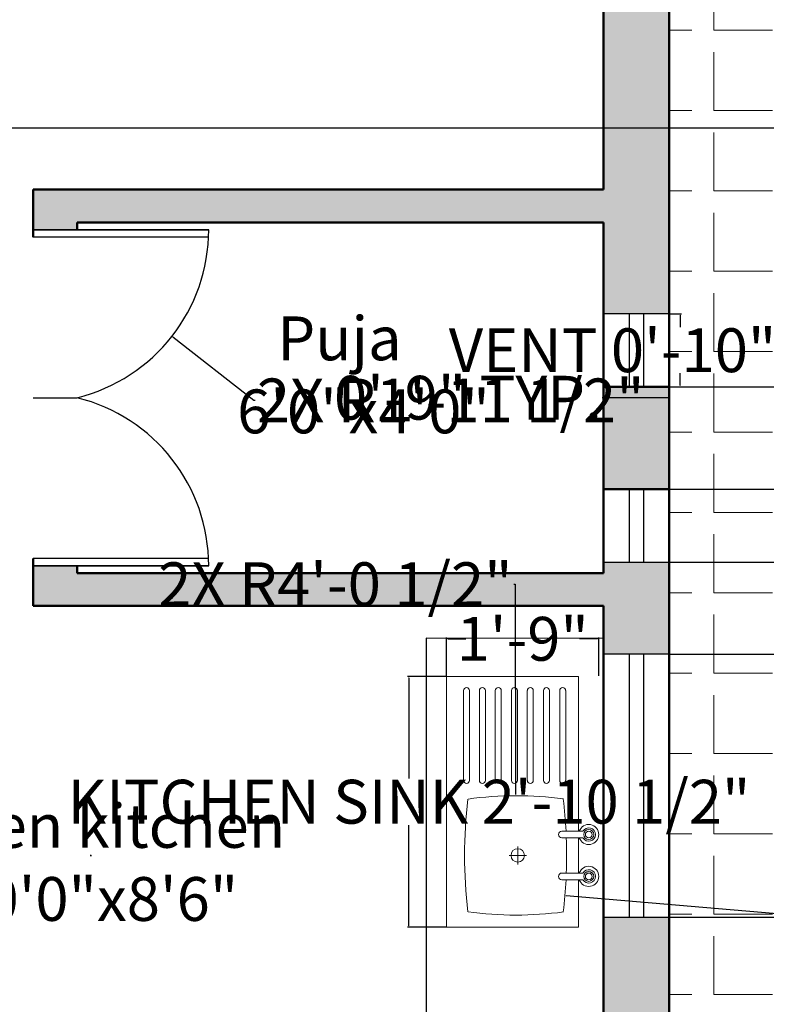
# Model space of a CAD drawing. Units: inches. Extents: x 1601 to 2080, y 5000 to 5589.
# Tile 5 of 11: x 1874 to 1976, y 5125 to 5259. Entities that reach past the tile are written whole.
import ezdxf

# ---------------------------------------------------------------- set-up
doc = ezdxf.new("R2010")
doc.units = ezdxf.units.IN
doc.header["$MEASUREMENT"] = 0
for name, color, linetype, lineweight in [('A-ANNO-DIMS', 2, 'Continuous', 18), ('A-AREA-IDEN', 7, 'Continuous', 25), ('A-COLS', 7, 'Continuous', 50), ('A-COLS-PATT', 18, 'Continuous', 13), ('A-DOOR', 3, 'Continuous', 25), ('A-FLOR-CASE', 8, 'Continuous', 25), ('A-FLOR-FIXT', 7, 'Continuous', 18), ('A-FLOR-PATT', 8, 'Continuous', 13), ('A-GLAZ', 4, 'Continuous', 25), ('A-WALL', 7, 'Continuous', 50), ('A-WALL-PATT', 241, 'Continuous', 13)]:
    doc.layers.add(name, color=color, linetype=linetype, lineweight=lineweight)
doc.styles.get("Standard").update_dxf_attribs({"font": 'arial.ttf'})
doc.dimstyles.get("Standard").update_dxf_attribs({"dimtxt": 6, "dimasz": 0.18, "dimexe": 0.18, "dimexo": 0.0625, "dimgap": 0.09, "dimtad": 0, "dimtih": 1, "dimtoh": 1, "dimdec": 1, "dimzin": 0, "dimdsep": 46, "dimlunit": 3, "dimtxsty": 'Standard', "dimcen": 0.09, "dimadec": 0, "dimazin": 0, "dimtfac": 1, "dimtdec": 1, "dimtofl": 0, "dimtmove": 0, "dimatfit": 3, "dimfxl": 1, "dimtolj": 1, "dimtzin": 0, "dimarcsym": 0})

# ---------------------------------------------------------------- blocks, each defined once
blk = doc.blocks.new('A$C799204C7')
for p, q in [((0, 34.2), (17.99, 34.2)), ((0, 0), (0, 34.2)), ((17.99, 13.08), (17.99, 34.2)), ((2.32, 20.01), (2.32, 32.27)), ((3.13, 20.01), (3.13, 32.27)), ((4.48, 20.01), (4.48, 32.27)), ((5.29, 20.01), (5.29, 32.27)), ((6.64, 20.01), (6.64, 32.27)), ((7.45, 20.01), (7.45, 32.27)), ((8.85, 20.01), (8.85, 32.27)), ((9.66, 20.01), (9.66, 32.27)), ((11.01, 20.01), (11.01, 32.27)), ((11.82, 20.01), (11.82, 32.27)), ((13.22, 20.01), (13.22, 32.27)), ((14.03, 20.01), (14.03, 32.27)), ((15.42, 20.01), (15.42, 32.27)), ((16.24, 20.01), (16.24, 32.27)), ((18.59, 13.08), (15.71, 13.08)), ((15.71, 12.17), (18.59, 12.17)), ((17.99, 7.36), (17.99, 12.17)), ((9.73, 11), (9.73, 8.54)), ((8.52, 9.77), (10.9, 9.77)), ((18.59, 7.36), (15.71, 7.36)), ((15.71, 6.45), (18.59, 6.45)), ((17.99, 0), (17.99, 6.45)), ((0, 0), (17.99, 0))]:
    blk.add_line(p, q)
for centre, radius in [((19.38, 12.62), 0.684), ((19.38, 12.62), 0.456), ((9.7, 9.77), 0.916), ((19.38, 6.91), 0.684), ((19.38, 6.91), 0.456)]:
    blk.add_circle(centre, radius)
for centre, radius, start, end in [((2.72, 32.27), 0.407, 0, 180), ((4.88, 32.27), 0.407, 0, 180), ((7.05, 32.27), 0.407, 0, 180), ((9.25, 32.27), 0.407, 0, 180), ((11.42, 32.27), 0.407, 0, 180), ((13.62, 32.27), 0.407, 0, 180), ((15.83, 32.27), 0.407, 0, 180), ((2.72, 20.01), 0.407, 180, 0), ((4.88, 20.01), 0.407, 180, 0), ((7.05, 20.01), 0.407, 180, 0), ((9.25, 20.01), 0.407, 180, 0), ((11.42, 20.01), 0.407, 180, 0), ((13.62, 20.01), 0.407, 180, 0), ((15.83, 20.01), 0.407, 180, 0), ((9.53, -30.19), 48.1, 82.3437, 97.8966), ((67.33, 9.77), 64.88, 173.1952, 186.8048), ((-48.51, 9.77), 64.88, 2.9208, 6.8048), ((19.38, 12.62), 1.37, 199.6514, 160.3603), ((19.38, 12.62), 0.911, 210.3431, 149.7554), ((15.71, 12.62), 0.456, 90, 270), ((-48.51, 9.77), 64.88, 357.8723, 2.115), ((19.38, 6.91), 1.37, 199.6514, 160.3603), ((15.71, 6.91), 0.456, 90, 270), ((19.38, 6.91), 0.911, 210.3431, 149.7554), ((-48.51, 9.77), 64.88, 353.1952, 357.0665), ((9.53, 49.73), 48.1, 262.1034, 277.6563)]:
    blk.add_arc(centre, radius, start, end)
blk = doc.blocks.new('WINDOW-36IN')
for p, q in [((0, 9), (0, 0)), ((36, 9), (0, 9)), ((36, 0), (36, 9)), ((36, 5.5), (0, 5.5)), ((0, 3.5), (36, 3.5)), ((0, 0), (36, 0))]:
    blk.add_line(p, q)
blk = doc.blocks.new('VENT-10IN')
for p, q in [((0, 10), (0, 0)), ((3.5, 10), (3.5, 0)), ((5.5, 0), (5.5, 10)), ((9, 0), (9, 10)), ((0, 0), (9, 0))]:
    blk.add_line(p, q)
blk = doc.blocks.new('*D33')
at = {"layer": 'A-ANNO-DIMS', "color": 0, "lineweight": -2, "transparency": 16777216}
for p, q in [((1962.97, 5219.2), (1964.59, 5219.2)), ((1964.41, 5219.02), (1964.41, 5217.35)), ((1964.41, 5209.38), (1964.41, 5211.04)), ((1962.97, 5209.2), (1964.59, 5209.2))]:
    blk.add_line(p, q, dxfattribs=at)
at = {"layer": 'A-ANNO-DIMS', "color": 0, "transparency": 16777216}
for points in [[(1964.38, 5219.02), (1964.44, 5219.02), (1964.41, 5219.2)], [(1964.38, 5209.38), (1964.44, 5209.38), (1964.41, 5209.2)]]:
    blk.add_solid(points, dxfattribs=at)
at = {"layer": 'Defpoints', "color": 0, "transparency": 16777216}
for p in [(1962.91, 5219.2), (1962.91, 5209.2), (1964.41, 5209.2)]:
    blk.add_point(p, dxfattribs=at)
at = {"layer": 'A-ANNO-DIMS', "color": 0, "transparency": 16777216, "insert": (1964.41, 5214.2), "char_height": 6, "attachment_point": 5}
blk.add_mtext('\\A1;VENT 0\'-10" TYP.', dxfattribs=at)
blk = doc.blocks.new('*D34')
at = {"layer": 'A-ANNO-DIMS', "color": 0, "lineweight": -2, "transparency": 16777216}
for p, q in [((1953.91, 5209.13), (1953.91, 5207.52)), ((1962.91, 5209.13), (1962.91, 5207.52)), ((1953.91, 5207.7), (1953.73, 5207.7)), ((1962.73, 5207.7), (1954.09, 5207.7))]:
    blk.add_line(p, q, dxfattribs=at)
at = {"layer": 'A-ANNO-DIMS', "color": 0, "transparency": 16777216}
for points in [[(1954.09, 5207.73), (1954.09, 5207.67), (1953.91, 5207.7)], [(1962.73, 5207.73), (1962.73, 5207.67), (1962.91, 5207.7)]]:
    blk.add_solid(points, dxfattribs=at)
at = {"layer": 'Defpoints', "color": 0, "transparency": 16777216}
for p in [(1953.91, 5209.2), (1962.91, 5209.2), (1953.91, 5207.7)]:
    blk.add_point(p, dxfattribs=at)
at = {"layer": 'A-ANNO-DIMS', "color": 0, "transparency": 16777216, "insert": (1935.35, 5207.7), "char_height": 6, "attachment_point": 5}
blk.add_mtext('\\A1;0\'-9" TYP.', dxfattribs=at)
blk = doc.blocks.new('*D35')
at = {"layer": 'A-ANNO-DIMS', "color": 0, "lineweight": -2, "transparency": 16777216}
for p, q in [((1932.38, 5169.56), (1927.11, 5169.56)), ((1927.29, 5169.38), (1927.29, 5155.59)), ((1927.29, 5135.43), (1927.29, 5149.21)), ((1932.38, 5135.25), (1927.11, 5135.25))]:
    blk.add_line(p, q, dxfattribs=at)
at = {"layer": 'A-ANNO-DIMS', "color": 0, "transparency": 16777216}
for points in [[(1927.26, 5169.38), (1927.32, 5169.38), (1927.29, 5169.56)], [(1927.26, 5135.43), (1927.32, 5135.43), (1927.29, 5135.25)]]:
    blk.add_solid(points, dxfattribs=at)
at = {"layer": 'Defpoints', "color": 0, "transparency": 16777216}
for p in [(1927.29, 5169.56), (1932.44, 5169.56), (1932.44, 5135.25)]:
    blk.add_point(p, dxfattribs=at)
at = {"layer": 'A-ANNO-DIMS', "color": 0, "transparency": 16777216, "insert": (1927.29, 5152.4), "char_height": 6, "attachment_point": 5}
blk.add_mtext('\\A1;KITCHEN SINK 2\'-10 1/2"', dxfattribs=at)
blk = doc.blocks.new('*D36')
at = {"layer": 'A-ANNO-DIMS', "color": 0, "lineweight": -2, "transparency": 16777216}
for p, q in [((1932.44, 5169.62), (1932.44, 5174.88)), ((1932.62, 5174.7), (1935.06, 5174.7)), ((1953.07, 5174.7), (1950.63, 5174.7)), ((1953.25, 5169.62), (1953.25, 5174.88))]:
    blk.add_line(p, q, dxfattribs=at)
at = {"layer": 'A-ANNO-DIMS', "color": 0, "transparency": 16777216}
for points in [[(1932.62, 5174.73), (1932.62, 5174.67), (1932.44, 5174.7)], [(1953.07, 5174.73), (1953.07, 5174.67), (1953.25, 5174.7)]]:
    blk.add_solid(points, dxfattribs=at)
at = {"layer": 'Defpoints', "color": 0, "transparency": 16777216}
for p in [(1953.25, 5174.7), (1932.44, 5169.56), (1953.25, 5169.56)]:
    blk.add_point(p, dxfattribs=at)
at = {"layer": 'A-ANNO-DIMS', "color": 0, "transparency": 16777216, "insert": (1942.85, 5174.7), "char_height": 6, "attachment_point": 5}
blk.add_mtext('\\A1;1\'-9"', dxfattribs=at)
blk = doc.blocks.new('*D50')
at = {"layer": 'A-ANNO-DIMS', "color": 0, "lineweight": -2, "transparency": 16777216}
for p, q in [((1962.97, 5136.6), (2047.44, 5136.6)), ((2047.26, 5136.42), (2047.26, 5106.29)), ((2047.26, 5069.88), (2047.26, 5100.01)), ((1962.97, 5069.7), (2047.44, 5069.7))]:
    blk.add_line(p, q, dxfattribs=at)
at = {"layer": 'A-ANNO-DIMS', "color": 0, "transparency": 16777216}
for points in [[(2047.23, 5136.42), (2047.29, 5136.42), (2047.26, 5136.6)], [(2047.23, 5069.88), (2047.29, 5069.88), (2047.26, 5069.7)]]:
    blk.add_solid(points, dxfattribs=at)
at = {"layer": 'Defpoints', "color": 0, "transparency": 16777216}
for p in [(1962.91, 5136.6), (2047.26, 5136.6), (1962.91, 5069.7)]:
    blk.add_point(p, dxfattribs=at)
at = {"layer": 'A-ANNO-DIMS', "color": 0, "transparency": 16777216, "insert": (2047.26, 5103.15), "char_height": 6, "attachment_point": 5}
blk.add_mtext('\\A1;5\'-7"', dxfattribs=at)
blk = doc.blocks.new('*D54')
at = {"layer": 'A-ANNO-DIMS', "color": 0, "lineweight": -2, "transparency": 16777216}
for p, q in [((1962.97, 5209.2), (2047.44, 5209.2)), ((2047.26, 5209.02), (2047.26, 5205.3)), ((2047.26, 5195.38), (2047.26, 5199.09)), ((1962.97, 5195.2), (2047.44, 5195.2))]:
    blk.add_line(p, q, dxfattribs=at)
at = {"layer": 'A-ANNO-DIMS', "color": 0, "transparency": 16777216}
for points in [[(2047.23, 5209.02), (2047.29, 5209.02), (2047.26, 5209.2)], [(2047.23, 5195.38), (2047.29, 5195.38), (2047.26, 5195.2)]]:
    blk.add_solid(points, dxfattribs=at)
at = {"layer": 'Defpoints', "color": 0, "transparency": 16777216}
for p in [(1962.91, 5209.2), (2047.26, 5209.2), (1962.91, 5195.2)]:
    blk.add_point(p, dxfattribs=at)
at = {"layer": 'A-ANNO-DIMS', "color": 0, "transparency": 16777216, "insert": (2047.26, 5202.2), "char_height": 6, "attachment_point": 5}
blk.add_mtext('\\A1;1\'-2"', dxfattribs=at)
blk = doc.blocks.new('*D55')
at = {"layer": 'A-ANNO-DIMS', "color": 0, "lineweight": -2, "transparency": 16777216}
for p, q in [((1962.97, 5185.2), (2047.44, 5185.2)), ((2047.26, 5185.02), (2047.26, 5182.09)), ((2047.26, 5172.78), (2047.26, 5175.71)), ((1962.97, 5172.6), (2047.44, 5172.6))]:
    blk.add_line(p, q, dxfattribs=at)
at = {"layer": 'A-ANNO-DIMS', "color": 0, "transparency": 16777216}
for points in [[(2047.23, 5185.02), (2047.29, 5185.02), (2047.26, 5185.2)], [(2047.23, 5172.78), (2047.29, 5172.78), (2047.26, 5172.6)]]:
    blk.add_solid(points, dxfattribs=at)
at = {"layer": 'Defpoints', "color": 0, "transparency": 16777216}
for p in [(1962.91, 5185.2), (2047.26, 5185.2), (1962.91, 5172.6)]:
    blk.add_point(p, dxfattribs=at)
at = {"layer": 'A-ANNO-DIMS', "color": 0, "transparency": 16777216, "insert": (2047.26, 5178.9), "char_height": 6, "attachment_point": 5}
blk.add_mtext('\\A1;1\'-0 1/2"', dxfattribs=at)
blk = doc.blocks.new('*D56')
at = {"layer": 'A-ANNO-DIMS', "color": 0, "lineweight": -2, "transparency": 16777216}
for p, q in [((1833.97, 5300.2), (2047.44, 5300.2)), ((2047.26, 5300.02), (2047.26, 5275.61)), ((2047.26, 5244.82), (2047.26, 5269.23)), ((1833.97, 5244.64), (2047.44, 5244.64))]:
    blk.add_line(p, q, dxfattribs=at)
at = {"layer": 'A-ANNO-DIMS', "color": 0, "transparency": 16777216}
for points in [[(2047.23, 5300.02), (2047.29, 5300.02), (2047.26, 5300.2)], [(2047.23, 5244.82), (2047.29, 5244.82), (2047.26, 5244.64)]]:
    blk.add_solid(points, dxfattribs=at)
at = {"layer": 'Defpoints', "color": 0, "transparency": 16777216}
for p in [(1833.91, 5300.2), (2047.26, 5300.2), (1833.91, 5244.64)]:
    blk.add_point(p, dxfattribs=at)
at = {"layer": 'A-ANNO-DIMS', "color": 0, "transparency": 16777216, "insert": (2047.26, 5272.42), "char_height": 6, "attachment_point": 5}
blk.add_mtext('\\A1;4\'-7 1/2"', dxfattribs=at)
blk = doc.blocks.new('*D59')
at = {"layer": 'A-ANNO-DIMS', "color": 0, "lineweight": -2, "transparency": 16777216}
for p, q in [((1876.12, 5230.7), (1876.3, 5230.7)), ((1876.21, 5230.61), (1876.21, 5230.79)), ((1906.07, 5207.33), (1895.01, 5215.98)), ((1906.25, 5207.33), (1906.07, 5207.33))]:
    blk.add_line(p, q, dxfattribs=at)
at = {"layer": 'A-ANNO-DIMS', "color": 0, "transparency": 16777216}
blk.add_solid([(1895.03, 5216.01), (1895, 5215.96), (1894.87, 5216.09)], dxfattribs=at)
at = {"layer": 'Defpoints', "color": 0, "transparency": 16777216}
for p in [(1876.21, 5230.7), (1894.87, 5216.09)]:
    blk.add_point(p, dxfattribs=at)
at = {"layer": 'A-ANNO-DIMS', "color": 0, "transparency": 16777216, "insert": (1933, 5207.33), "char_height": 6, "attachment_point": 5}
blk.add_mtext('\\A1;2X R1\'-11 1/2"', dxfattribs=at)
blk = doc.blocks.new('*D63')
at = {"layer": 'A-ANNO-DIMS', "color": 0, "lineweight": -2, "transparency": 16777216}
for p, q in [((1883.68, 5145.05), (1883.86, 5145.05)), ((1883.77, 5144.96), (1883.77, 5145.14)), ((1987.53, 5136.21), (1948.8, 5139.51))]:
    blk.add_line(p, q, dxfattribs=at)
at = {"layer": 'A-ANNO-DIMS', "color": 0, "transparency": 16777216}
blk.add_solid([(1948.8, 5139.54), (1948.8, 5139.48), (1948.62, 5139.53)], dxfattribs=at)
at = {"layer": 'Defpoints', "color": 0, "transparency": 16777216}
for p in [(1883.77, 5145.05), (1948.62, 5139.53)]:
    blk.add_point(p, dxfattribs=at)
at = {"layer": 'A-ANNO-DIMS', "color": 0, "transparency": 16777216, "insert": (2004.91, 5136.21), "char_height": 6, "attachment_point": 5}
blk.add_mtext('\\A1;3X R5\'-5"', dxfattribs=at)
blk = doc.blocks.new('*D64')
at = {"layer": 'A-ANNO-DIMS', "color": 0, "lineweight": -2, "transparency": 16777216}
for p, q in [((1941.65, 5182.17), (1941.83, 5182.17)), ((1941.83, 5182.17), (1941.89, 5153.4)), ((1941.91, 5104.96), (1942.09, 5104.96)), ((1942, 5104.87), (1942, 5105.05))]:
    blk.add_line(p, q, dxfattribs=at)
at = {"layer": 'A-ANNO-DIMS', "color": 0, "transparency": 16777216}
blk.add_solid([(1941.92, 5153.4), (1941.86, 5153.4), (1941.89, 5153.22)], dxfattribs=at)
at = {"layer": 'Defpoints', "color": 0, "transparency": 16777216}
for p in [(1941.89, 5153.22), (1942, 5104.96)]:
    blk.add_point(p, dxfattribs=at)
at = {"layer": 'A-ANNO-DIMS', "color": 0, "transparency": 16777216, "insert": (1917.23, 5182.17), "char_height": 6, "attachment_point": 5}
blk.add_mtext('\\A1;2X R4\'-0 1/2"', dxfattribs=at)

msp = doc.modelspace()

# ---------------------------------------------------------------- hatches: boundary and pattern name
at = {"layer": 'A-COLS-PATT'}
h = msp.add_hatch(color=256, dxfattribs=at)
h.dxf.hatch_style = 1
h.paths.add_polyline_path([(1702.41, 5431.2), (1688.41, 5431.2), (1688.41, 5422.2), (1702.41, 5422.2)])
h.paths.add_polyline_path([(1836.17, 5431.2), (1822.17, 5431.2), (1822.17, 5422.2), (1836.17, 5422.2)])
h.paths.add_polyline_path([(1962.91, 5431.2), (1948.91, 5431.2), (1948.91, 5422.2), (1962.91, 5422.2)])
h.paths.add_polyline_path([(1697.41, 5314.2), (1688.41, 5314.2), (1688.41, 5300.2), (1697.41, 5300.2)])
h.paths.add_polyline_path([(1833.91, 5314.2), (1824.91, 5314.2), (1824.91, 5300.2), (1833.91, 5300.2)])
h.paths.add_polyline_path([(1962.91, 5314.2), (1953.91, 5314.2), (1953.91, 5300.2), (1962.91, 5300.2)])
h.paths.add_polyline_path([(1697.41, 5209.2), (1688.41, 5209.2), (1688.41, 5195.2), (1697.41, 5195.2)])
h.paths.add_polyline_path([(1833.91, 5209.2), (1824.91, 5209.2), (1824.91, 5195.2), (1833.91, 5195.2)])
h.paths.add_polyline_path([(1962.91, 5209.2), (1953.91, 5209.2), (1953.91, 5195.2), (1962.91, 5195.2)])
h.paths.add_polyline_path([(1697.41, 5083.7), (1688.41, 5083.7), (1688.41, 5069.7), (1697.41, 5069.7)])
h.paths.add_polyline_path([(1833.91, 5078.7), (1819.91, 5078.7), (1819.91, 5069.7), (1833.91, 5069.7)])
h.paths.add_polyline_path([(1962.91, 5078.7), (1948.91, 5078.7), (1948.91, 5069.7), (1962.91, 5069.7)])
at = {"layer": 'A-FLOR-PATT'}
h = msp.add_hatch(dxfattribs=at)
h.set_pattern_fill('ANGLE', color=256, scale=40)
h.set_pattern_definition([(0, (0, 0), (0, 11), [8, -3]), (90, (0, 0), (-11, 7e-16), [8, -3])])
h.paths.add_polyline_path([(2022.91, 5509.2), (1941.91, 5509.2), (1911.91, 5509.2), (1864.41, 5509.2), (1864.41, 5489.7), (1868.54, 5489.7, -0.022155), (1868.52, 5490.01, -1), (1875.53, 5490.01, -0.956651), (1868.54, 5489.7), (1864.41, 5489.7), (1864.41, 5470.2), (1794.41, 5470.2), (1794.41, 5431.2), (1811.95, 5431.2), (1911.91, 5431.2), (1941.91, 5431.2), (1942.91, 5431.2), (1945.91, 5431.2), (1948.91, 5431.2), (1962.91, 5431.2), (1962.91, 5415.29), (1962.91, 5385.29), (1962.91, 5384.29), (1962.91, 5381.29), (1962.91, 5333.29), (1962.91, 5069.7), (2022.91, 5069.7)])
h.paths.add_polyline_path([(2000.28, 5267.55), (2000.28, 5367.64), (1987.91, 5367.64), (1987.91, 5267.55)], flags=24)
h.paths.add_polyline_path([(1879.42, 5455.52), (1969.04, 5455.52), (1969.04, 5467.88), (1879.42, 5467.88)], flags=24)
at = {"layer": 'A-WALL-PATT'}
h = msp.add_hatch(color=256, dxfattribs=at)
h.dxf.hatch_style = 1
h.paths.add_polyline_path([(1763.95, 5431.2), (1702.41, 5431.2), (1702.41, 5422.2), (1763.95, 5422.2)])
h.paths.add_polyline_path([(1697.41, 5422.2), (1688.41, 5422.2), (1688.41, 5314.2), (1697.41, 5314.2)])
h.paths.add_polyline_path([(1740.41, 5314.2), (1697.41, 5314.2), (1697.41, 5309.7), (1740.41, 5309.7)], flags=17)
h.paths.add_polyline_path([(1822.17, 5431.2), (1811.95, 5431.2), (1811.95, 5422.2), (1822.17, 5422.2)])
h.paths.add_polyline_path([(1845.52, 5431.2), (1836.17, 5431.2), (1836.17, 5422.2), (1845.52, 5422.2)])
h.paths.add_polyline_path([(1910.91, 5431.2), (1881.52, 5431.2), (1881.52, 5422.2), (1910.91, 5422.2)])
h.paths.add_polyline_path([(1948.91, 5431.2), (1945.91, 5431.2), (1942.91, 5431.2), (1942.91, 5422.2), (1948.91, 5422.2)])
h.paths.add_polyline_path([(1962.91, 5422.2), (1953.91, 5422.2), (1953.91, 5416.29), (1962.91, 5416.29)])
h.paths.add_polyline_path([(1962.91, 5384.29), (1953.91, 5384.29), (1953.91, 5381.29), (1962.91, 5381.29)])
h.paths.add_polyline_path([(1962.91, 5333.29), (1953.91, 5333.29), (1953.91, 5314.2), (1962.91, 5314.2)])
h.paths.add_polyline_path([(1962.91, 5300.2), (1953.91, 5300.2), (1953.91, 5236.2), (1875.91, 5236.2), (1875.91, 5230.7), (1881.91, 5230.7), (1881.91, 5231.7), (1953.91, 5231.7), (1953.91, 5219.2), (1962.91, 5219.2)])
h.paths.add_polyline_path([(1962.91, 5185.2), (1953.91, 5185.2), (1953.91, 5183.7), (1881.91, 5183.7), (1881.91, 5184.7), (1875.91, 5184.7), (1875.91, 5183.7), (1875.91, 5179.2), (1953.91, 5179.2), (1953.91, 5172.6), (1962.91, 5172.6)])
h.paths.add_polyline_path([(1962.91, 5136.6), (1953.91, 5136.6), (1953.91, 5078.7), (1962.91, 5078.7)])
h.paths.add_polyline_path([(1948.91, 5078.7), (1833.91, 5078.7), (1833.91, 5069.7), (1948.91, 5069.7)])
h.paths.add_polyline_path([(1833.91, 5195.2), (1829.41, 5195.2), (1829.41, 5078.7), (1833.91, 5078.7)])
h.paths.add_polyline_path([(1819.91, 5078.7), (1813.58, 5078.7), (1813.58, 5069.7), (1819.91, 5069.7)])
h.paths.add_polyline_path([(1765.58, 5078.7), (1697.41, 5078.7), (1697.41, 5069.7), (1765.58, 5069.7)])
h.paths.add_polyline_path([(1697.41, 5195.2), (1688.41, 5195.2), (1688.41, 5083.7), (1697.41, 5083.7)])
h.paths.add_polyline_path([(1740.41, 5209.2), (1697.41, 5209.2), (1697.41, 5204.7), (1740.41, 5204.7)], flags=17)
h.paths.add_polyline_path([(1787.91, 5209.2), (1779.91, 5209.2), (1779.91, 5309.7), (1787.91, 5309.7), (1787.91, 5314.2), (1772.41, 5314.2), (1772.41, 5309.7), (1775.41, 5309.7), (1775.41, 5261.7), (1697.41, 5261.7), (1697.41, 5273.07), (1688.41, 5273.07), (1688.41, 5242.37), (1697.41, 5242.37), (1697.41, 5257.2), (1775.41, 5257.2), (1775.41, 5209.2), (1772.41, 5209.2), (1772.41, 5204.7), (1775.41, 5204.7), (1787.91, 5204.7)])
h.paths.add_polyline_path([(1697.41, 5218.37), (1688.41, 5218.37), (1688.41, 5209.2), (1697.41, 5209.2)], flags=17)
h.paths.add_polyline_path([(1833.91, 5422.2), (1829.41, 5422.2), (1829.41, 5314.2), (1833.91, 5314.2)])
h.paths.add_polyline_path([(1697.41, 5300.2), (1688.41, 5300.2), (1688.41, 5297.07), (1697.41, 5297.07)], flags=17)

# ---------------------------------------------------------------- linework, layer by layer
at = {"layer": 'A-COLS'}
for p, q in [((1953.91, 5195.2), (1953.91, 5209.2)), ((1953.91, 5209.2), (1962.91, 5209.2)), ((1962.91, 5209.2), (1962.91, 5195.2)), ((1962.91, 5195.2), (1953.91, 5195.2))]:
    msp.add_line(p, q, dxfattribs=at)
at = {"layer": 'A-DOOR'}
for p, q in [((1875.91, 5230.7), (1899.91, 5230.7)), ((1899.91, 5230.7), (1875.91, 5230.7)), ((1875.91, 5230.7), (1875.91, 5229.7)), ((1875.91, 5229.7), (1875.91, 5230.7)), ((1899.91, 5229.7), (1875.91, 5229.7)), ((1875.91, 5207.7), (1881.91, 5207.7)), ((1875.91, 5184.7), (1875.91, 5185.7)), ((1899.91, 5185.7), (1875.91, 5185.7)), ((1875.91, 5184.7), (1899.91, 5184.7)), ((1899.91, 5184.7), (1875.91, 5184.7))]:
    msp.add_line(p, q, dxfattribs=at)
for centre, start, end in [((1876.21, 5230.7), 283.9059, 360), ((1876.21, 5184.7), 0, 76.0941)]:
    msp.add_arc(centre, 23.69, start, end, dxfattribs=at)
at = {"layer": 'A-FLOR-CASE'}
for p, q in [((1953.91, 5174.73), (1929.65, 5174.81)), ((1929.65, 5174.81), (1929.65, 5106.95))]:
    msp.add_line(p, q, dxfattribs=at)
at = {"layer": 'A-WALL'}
for p, q in [((1962.91, 5385.29), (1962.91, 5069.7)), ((1953.91, 5384.29), (1953.91, 5236.2)), ((1875.91, 5236.2), (1875.91, 5229.7)), ((1875.91, 5236.2), (1953.91, 5236.2)), ((1881.91, 5231.7), (1881.91, 5230.7)), ((1881.91, 5231.7), (1953.91, 5231.7)), ((1953.91, 5231.7), (1953.91, 5183.7)), ((1875.91, 5185.7), (1875.91, 5179.2)), ((1875.91, 5183.7), (1875.91, 5184.7)), ((1881.91, 5184.7), (1881.91, 5183.7)), ((1881.91, 5183.7), (1953.91, 5183.7)), ((1875.91, 5179.2), (1953.91, 5179.2)), ((1953.91, 5179.2), (1953.91, 5078.7))]:
    msp.add_line(p, q, dxfattribs=at)

# ---------------------------------------------------------------- block references
at = {"layer": 'A-FLOR-FIXT', "xscale": 1.0032, "yscale": 1.0032, "zscale": 1.0032}
msp.add_blockref('A$C799204C7', (1932.44, 5135.25), dxfattribs=at)
at = {"layer": 'A-GLAZ'}
for name, p, rotation in [('VENT-10IN', (1962.91, 5219.2), 180), ('WINDOW-36IN', (1953.91, 5172.6), 270.0000000000027)]:
    msp.add_blockref(name, p, dxfattribs=dict(at, rotation=rotation))
msp.add_blockref('VENT-10IN', (1953.91, 5185.2), dxfattribs=at)

# ---------------------------------------------------------------- texts
at = {"layer": 'A-AREA-IDEN', "char_height": 6, "attachment_point": 1}
for s, width, insert in [('   Puja\\P6\'0"x4\'0"', 39.9171, (1903.79, 5218.83)), ('Open kitchen\\P   10\'0"x8\'6"', 60.0959, (1859.33, 5152.09))]:
    msp.add_mtext_dynamic_manual_height_columns(s, width=width, gutter_width=30, heights=[0], dxfattribs=dict(at, insert=insert))

# ---------------------------------------------------------------- dimensions: what is measured, and where the dimension line sits
at = {"layer": 'A-ANNO-DIMS'}
for base, p1, p2, picture, middle in [((2047.26, 5300.2), (1833.91, 5244.64), (1833.91, 5300.2), '*D56', (2047.26, 5272.42)), ((2047.26, 5209.2), (1962.91, 5195.2), (1962.91, 5209.2), '*D54', (2047.26, 5202.2)), ((2047.26, 5185.2), (1962.91, 5172.6), (1962.91, 5185.2), '*D55', (2047.26, 5178.9)), ((2047.26, 5136.6), (1962.91, 5069.7), (1962.91, 5136.6), '*D50', (2047.26, 5103.15))]:
    dim = msp.add_linear_dim(base=base, p1=p1, p2=p2, angle=90, dimstyle='Standard', override={"dimdec": 1, "dimlfac": 1, "dimrnd": 0, "dimzin": 1, "dimdsep": 46, "dimlunit": 4, "dimfrac": 2}, dxfattribs=at)
    dim.commit()
    dim.dimension.update_dxf_attribs({"geometry": picture, "text_midpoint": middle})
for center, mpoint, text, picture, middle in [((1876.21, 5230.7), (1894.87, 5216.09), '2X <>', '*D59', (1933, 5207.33)), ((1942, 5104.96), (1941.89, 5153.22), '2X <>', '*D64', (1917.23, 5182.17)), ((1883.77, 5145.05), (1948.62, 5139.53), '3X <>', '*D63', (1987.53, 5136.21))]:
    dim = msp.add_radius_dim(center=center, mpoint=mpoint, text=text, dimstyle='Standard', override={"dimdec": 1, "dimlfac": 1, "dimrnd": 0, "dimzin": 1, "dimdsep": 46, "dimlunit": 4, "dimfrac": 2}, dxfattribs=at)
    dim.commit()
    dim.dimension.update_dxf_attribs({"geometry": picture, "text_midpoint": middle, "dimtype": 164})
for base, p1, p2, angle, text, picture, middle in [((1964.41, 5209.2), (1962.91, 5219.2), (1962.91, 5209.2), 270, 'VENT <> TYP.', '*D33', (1964.41, 5214.2)), ((1953.91, 5207.7), (1962.91, 5209.2), (1953.91, 5209.2), 180, '<> TYP.', '*D34', (1935.35, 5207.7)), ((1927.29, 5169.56), (1932.44, 5135.25), (1932.44, 5169.56), 90, 'KITCHEN SINK <>', '*D35', (1927.29, 5152.4))]:
    dim = msp.add_linear_dim(base=base, p1=p1, p2=p2, angle=angle, text=text, dimstyle='Standard', override={"dimdec": 1, "dimlfac": 1, "dimrnd": 0, "dimzin": 1, "dimdsep": 46, "dimlunit": 4, "dimfrac": 2}, dxfattribs=at)
    dim.commit()
    dim.dimension.update_dxf_attribs({"geometry": picture, "text_midpoint": middle})
dim = msp.add_linear_dim(base=(1953.25, 5174.7), p1=(1932.44, 5169.56), p2=(1953.25, 5169.56), dimstyle='Standard', override={"dimdec": 1, "dimlfac": 1, "dimrnd": 0, "dimzin": 1, "dimdsep": 46, "dimlunit": 4, "dimfrac": 2}, dxfattribs=at)
dim.commit()
dim.dimension.update_dxf_attribs({"geometry": '*D36', "text_midpoint": (1942.85, 5174.7)})

doc.saveas('drawing.dxf')
